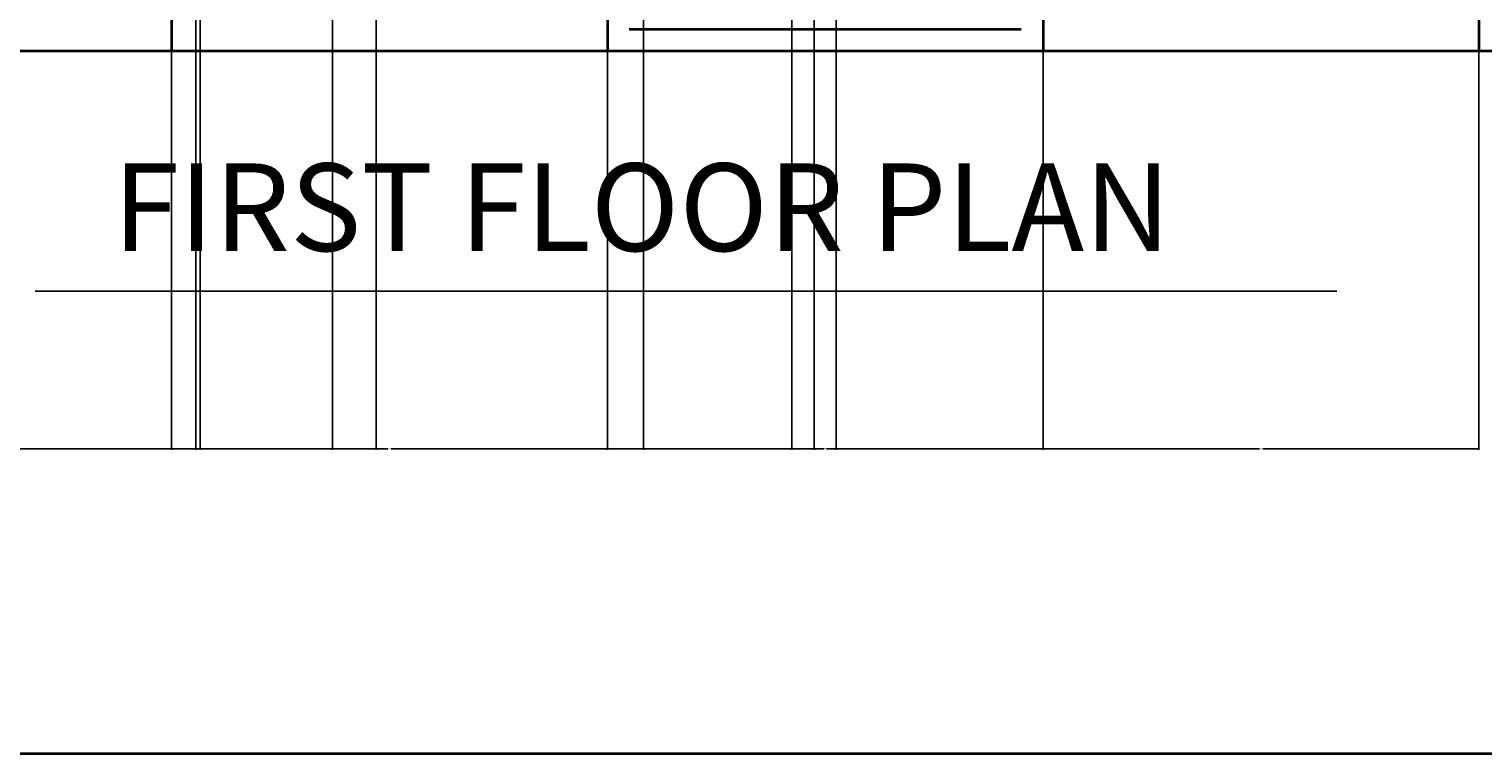
# Model space of a CAD drawing. Units: inches. Extents: x 1721 to 2510, y 1544 to 2360.
# Tile 2 of 10: x 1924 to 2222, y 1544 to 1693. Entities that reach past the tile are written whole.
import ezdxf

# ---------------------------------------------------------------- set-up
doc = ezdxf.new("R2010")
doc.units = ezdxf.units.IN
for name, color, linetype, lineweight in [('A-ANNO-DIMS', 2, 'Continuous', 18), ('A-ANNO-TEXT', 7, 'Continuous', 25), ('A-ANNO-TTLB', 7, 'Continuous', 35), ('A-WALL', 7, 'Continuous', 35)]:
    doc.layers.add(name, color=color, linetype=linetype, lineweight=lineweight)
doc.styles.get("Standard").update_dxf_attribs({"font": 'arial.ttf'})
doc.dimstyles.get("Standard").update_dxf_attribs({"dimtxt": 0.18, "dimasz": 0.18, "dimexe": 0.18, "dimexo": 0.0625, "dimgap": 0.09, "dimtad": 0, "dimtih": 1, "dimtoh": 1, "dimdec": 4, "dimzin": 0, "dimdsep": 46, "dimtxsty": 'Standard', "dimcen": 0.09, "dimadec": 0, "dimazin": 0, "dimtfac": 1, "dimtdec": 4, "dimtofl": 0, "dimtmove": 0, "dimatfit": 3, "dimfxl": 1, "dimtolj": 1, "dimtzin": 0, "dimarcsym": 0})

# ---------------------------------------------------------------- blocks, each defined once
blk = doc.blocks.new('*D42')
at = {"layer": 'A-ANNO-DIMS', "color": 0, "lineweight": -2, "transparency": 16777216}
for p, q in [((1798, 1688.57), (1798, 1606.75)), ((1953, 1688.57), (1953, 1606.75)), ((1798.18, 1606.93), (1875.22, 1606.93)), ((1952.82, 1606.93), (1875.78, 1606.93))]:
    blk.add_line(p, q, dxfattribs=at)
at = {"layer": 'A-ANNO-DIMS', "color": 0, "transparency": 16777216}
for points in [[(1798.18, 1606.96), (1798.18, 1606.9), (1798, 1606.93)], [(1952.82, 1606.96), (1952.82, 1606.9), (1953, 1606.93)]]:
    blk.add_solid(points, dxfattribs=at)
at = {"layer": 'Defpoints', "color": 0, "transparency": 16777216}
for p in [(1798, 1688.63), (1953, 1688.63), (1953, 1606.93)]:
    blk.add_point(p, dxfattribs=at)
at = {"layer": 'A-ANNO-DIMS', "color": 0, "transparency": 16777216, "insert": (1875.5, 1606.93), "char_height": 0.18, "attachment_point": 5}
blk.add_mtext('\\A1;155', dxfattribs=at)
blk = doc.blocks.new('*D43')
at = {"layer": 'A-ANNO-DIMS', "color": 0, "lineweight": -2, "transparency": 16777216}
for p, q in [((1953, 1688.57), (1953, 1606.75)), ((2042.5, 1688.57), (2042.5, 1606.75)), ((1953.18, 1606.93), (1997.43, 1606.93)), ((2042.32, 1606.93), (1998.08, 1606.93))]:
    blk.add_line(p, q, dxfattribs=at)
at = {"layer": 'A-ANNO-DIMS', "color": 0, "transparency": 16777216}
for points in [[(1953.18, 1606.96), (1953.18, 1606.9), (1953, 1606.93)], [(2042.32, 1606.96), (2042.32, 1606.9), (2042.5, 1606.93)]]:
    blk.add_solid(points, dxfattribs=at)
at = {"layer": 'Defpoints', "color": 0, "transparency": 16777216}
for p in [(1953, 1688.63), (2042.5, 1688.63), (2042.5, 1606.93)]:
    blk.add_point(p, dxfattribs=at)
at = {"layer": 'A-ANNO-DIMS', "color": 0, "transparency": 16777216, "insert": (1997.75, 1606.93), "char_height": 0.18, "attachment_point": 5}
blk.add_mtext('\\A1;89.5', dxfattribs=at)
blk = doc.blocks.new('*D44')
at = {"layer": 'A-ANNO-DIMS', "color": 0, "lineweight": -2, "transparency": 16777216}
for p, q in [((2042.5, 1688.57), (2042.5, 1606.75)), ((2132, 1688.57), (2132, 1606.75)), ((2042.68, 1606.93), (2086.93, 1606.93)), ((2131.82, 1606.93), (2087.58, 1606.93))]:
    blk.add_line(p, q, dxfattribs=at)
at = {"layer": 'A-ANNO-DIMS', "color": 0, "transparency": 16777216}
for points in [[(2042.68, 1606.96), (2042.68, 1606.9), (2042.5, 1606.93)], [(2131.82, 1606.96), (2131.82, 1606.9), (2132, 1606.93)]]:
    blk.add_solid(points, dxfattribs=at)
at = {"layer": 'Defpoints', "color": 0, "transparency": 16777216}
for p in [(2042.5, 1688.63), (2132, 1688.63), (2132, 1606.93)]:
    blk.add_point(p, dxfattribs=at)
at = {"layer": 'A-ANNO-DIMS', "color": 0, "transparency": 16777216, "insert": (2087.25, 1606.93), "char_height": 0.18, "attachment_point": 5}
blk.add_mtext('\\A1;89.5', dxfattribs=at)
blk = doc.blocks.new('*D45')
at = {"layer": 'A-ANNO-DIMS', "color": 0, "lineweight": -2, "transparency": 16777216}
for p, q in [((2132, 1688.57), (2132, 1606.75)), ((2221.5, 1688.57), (2221.5, 1606.75)), ((2132.18, 1606.93), (2176.43, 1606.93)), ((2221.32, 1606.93), (2177.08, 1606.93))]:
    blk.add_line(p, q, dxfattribs=at)
at = {"layer": 'A-ANNO-DIMS', "color": 0, "transparency": 16777216}
for points in [[(2132.18, 1606.96), (2132.18, 1606.9), (2132, 1606.93)], [(2221.32, 1606.96), (2221.32, 1606.9), (2221.5, 1606.93)]]:
    blk.add_solid(points, dxfattribs=at)
at = {"layer": 'Defpoints', "color": 0, "transparency": 16777216}
for p in [(2132, 1688.63), (2221.5, 1688.63), (2221.5, 1606.93)]:
    blk.add_point(p, dxfattribs=at)
at = {"layer": 'A-ANNO-DIMS', "color": 0, "transparency": 16777216, "insert": (2176.75, 1606.93), "char_height": 0.18, "attachment_point": 5}
blk.add_mtext('\\A1;89.5', dxfattribs=at)
blk = doc.blocks.new('*D62')
at = {"layer": 'A-ANNO-DIMS', "color": 0, "lineweight": -2, "transparency": 16777216}
for p, q in [((1957.99, 2252.88), (1957.99, 1606.75)), ((1986.02, 2252.88), (1986.02, 1606.75)), ((1958.17, 1606.93), (1971.61, 1606.93)), ((1985.84, 1606.93), (1972.4, 1606.93))]:
    blk.add_line(p, q, dxfattribs=at)
at = {"layer": 'A-ANNO-DIMS', "color": 0, "transparency": 16777216}
for points in [[(1958.17, 1606.96), (1958.17, 1606.9), (1957.99, 1606.93)], [(1985.84, 1606.96), (1985.84, 1606.9), (1986.02, 1606.93)]]:
    blk.add_solid(points, dxfattribs=at)
at = {"layer": 'Defpoints', "color": 0, "transparency": 16777216}
for p in [(1957.99, 2252.94), (1986.02, 2252.94), (1986.02, 1606.93)]:
    blk.add_point(p, dxfattribs=at)
at = {"layer": 'A-ANNO-DIMS', "color": 0, "transparency": 16777216, "insert": (1972.01, 1606.93), "char_height": 0.18, "attachment_point": 5}
blk.add_mtext('\\A1;28.03', dxfattribs=at)
blk = doc.blocks.new('*D63')
at = {"layer": 'A-ANNO-DIMS', "color": 0, "lineweight": -2, "transparency": 16777216}
for p, q in [((1958.89, 2116.38), (1958.89, 1606.75)), ((1995.05, 2116.38), (1995.05, 1606.75)), ((1959.07, 1606.93), (1976.58, 1606.93)), ((1994.87, 1606.93), (1977.36, 1606.93))]:
    blk.add_line(p, q, dxfattribs=at)
at = {"layer": 'A-ANNO-DIMS', "color": 0, "transparency": 16777216}
for points in [[(1959.07, 1606.96), (1959.07, 1606.9), (1958.89, 1606.93)], [(1994.87, 1606.96), (1994.87, 1606.9), (1995.05, 1606.93)]]:
    blk.add_solid(points, dxfattribs=at)
at = {"layer": 'Defpoints', "color": 0, "transparency": 16777216}
for p in [(1958.89, 2116.44), (1995.05, 2116.44), (1995.05, 1606.93)]:
    blk.add_point(p, dxfattribs=at)
at = {"layer": 'A-ANNO-DIMS', "color": 0, "transparency": 16777216, "insert": (1976.97, 1606.93), "char_height": 0.18, "attachment_point": 5}
blk.add_mtext('\\A1;36.16', dxfattribs=at)
blk = doc.blocks.new('*D64')
at = {"layer": 'A-ANNO-DIMS', "color": 0, "lineweight": -2, "transparency": 16777216}
for p, q in [((2049.89, 1986.57), (2049.89, 1606.75)), ((2080.39, 1986.57), (2080.39, 1606.75)), ((2050.07, 1606.93), (2064.81, 1606.93)), ((2080.21, 1606.93), (2065.46, 1606.93))]:
    blk.add_line(p, q, dxfattribs=at)
at = {"layer": 'A-ANNO-DIMS', "color": 0, "transparency": 16777216}
for points in [[(2050.07, 1606.96), (2050.07, 1606.9), (2049.89, 1606.93)], [(2080.21, 1606.96), (2080.21, 1606.9), (2080.39, 1606.93)]]:
    blk.add_solid(points, dxfattribs=at)
at = {"layer": 'Defpoints', "color": 0, "transparency": 16777216}
for p in [(2049.89, 1986.63), (2080.39, 1986.63), (2080.39, 1606.93)]:
    blk.add_point(p, dxfattribs=at)
at = {"layer": 'A-ANNO-DIMS', "color": 0, "transparency": 16777216, "insert": (2065.14, 1606.93), "char_height": 0.18, "attachment_point": 5}
blk.add_mtext('\\A1;30.5', dxfattribs=at)
blk = doc.blocks.new('*D65')
at = {"layer": 'A-ANNO-DIMS', "color": 0, "lineweight": -2, "transparency": 16777216}
for p, q in [((2085, 2116.38), (2085, 1606.75)), ((2089.5, 2116.38), (2089.5, 1606.75)), ((2085.18, 1606.93), (2086.99, 1606.93)), ((2089.32, 1606.93), (2087.51, 1606.93))]:
    blk.add_line(p, q, dxfattribs=at)
at = {"layer": 'A-ANNO-DIMS', "color": 0, "transparency": 16777216}
for points in [[(2085.18, 1606.96), (2085.18, 1606.9), (2085, 1606.93)], [(2089.32, 1606.96), (2089.32, 1606.9), (2089.5, 1606.93)]]:
    blk.add_solid(points, dxfattribs=at)
at = {"layer": 'Defpoints', "color": 0, "transparency": 16777216}
for p in [(2085, 2116.44), (2089.5, 2116.44), (2089.5, 1606.93)]:
    blk.add_point(p, dxfattribs=at)
at = {"layer": 'A-ANNO-DIMS', "color": 0, "transparency": 16777216, "insert": (2087.25, 1606.93), "char_height": 0.18, "attachment_point": 5}
blk.add_mtext('\\A1;4.5', dxfattribs=at)
blk = doc.blocks.new('*D67')
at = {"layer": 'A-ANNO-DIMS', "color": 0, "lineweight": -2, "transparency": 16777216}
for p, q in [((2042.44, 1725.13), (1765.42, 1725.13)), ((1765.6, 1724.95), (1765.6, 1707.06)), ((1765.6, 1688.81), (1765.6, 1706.7)), ((2042.44, 1688.63), (1765.42, 1688.63))]:
    blk.add_line(p, q, dxfattribs=at)
at = {"layer": 'A-ANNO-DIMS', "color": 0, "transparency": 16777216}
for points in [[(1765.57, 1724.95), (1765.63, 1724.95), (1765.6, 1725.13)], [(1765.57, 1688.81), (1765.63, 1688.81), (1765.6, 1688.63)]]:
    blk.add_solid(points, dxfattribs=at)
at = {"layer": 'Defpoints', "color": 0, "transparency": 16777216}
for p in [(1765.6, 1725.13), (2042.5, 1725.13), (2042.5, 1688.63)]:
    blk.add_point(p, dxfattribs=at)
at = {"layer": 'A-ANNO-DIMS', "color": 0, "transparency": 16777216, "insert": (1765.6, 1706.88), "char_height": 0.18, "attachment_point": 5}
blk.add_mtext('\\A1;36.5', dxfattribs=at)

msp = doc.modelspace()

# ---------------------------------------------------------------- linework, layer by layer
at = {"layer": 'A-ANNO-TEXT'}
msp.add_line((1924.9747, 1639.3297), (2192.2869, 1639.3297), dxfattribs=at)
at = {"layer": 'A-ANNO-TTLB'}
msp.add_lwpolyline([(1721.1268, 2360.2177), (2509.707, 2360.2177), (2509.707, 1544.3037), (1721.1268, 1544.3037)], close=True, dxfattribs=at)
at = {"layer": 'A-WALL'}
for p, q in [((1953.0024, 1829.1298), (1953.0024, 1688.6298)), ((2042.5024, 1725.1298), (2042.5024, 1688.6298)), ((2132.0024, 1725.1298), (2132.0024, 1688.6298)), ((2221.5024, 1725.1298), (2221.5024, 1688.6298)), ((2047.0024, 1693.1298), (2127.5024, 1693.1298)), ((1798.0024, 1688.6298), (2376.5024, 1688.6298))]:
    msp.add_line(p, q, dxfattribs=at)

# ---------------------------------------------------------------- texts
at = {"layer": 'A-ANNO-TEXT', "insert": (1940.9862, 1665.5549), "char_height": 18, "attachment_point": 1}
msp.add_mtext_dynamic_manual_height_columns('FIRST FLOOR PLAN', width=420.795796, gutter_width=12.5, heights=[0], dxfattribs=at)

# ---------------------------------------------------------------- dimensions: what is measured, and where the dimension line sits
at = {"layer": 'A-ANNO-DIMS'}
for base, p1, p2, override, picture, middle in [((1986.0213, 1606.9297), (1957.9903, 2252.9416), (1986.0213, 2252.9416), {"dimdec": 2, "dimlfac": 1, "dimrnd": 0, "dimzin": 0, "dimdsep": 46, "dimlunit": 2}, '*D62', (1972.0058, 1606.9297)), ((1995.0512, 1606.9297), (1958.8889, 2116.4416), (1995.0512, 2116.4416), {"dimdec": 2, "dimlfac": 1, "dimrnd": 0, "dimzin": 0, "dimdsep": 46, "dimlunit": 2}, '*D63', (1976.97, 1606.9297)), ((2089.5024, 1606.9297), (2085.0024, 2116.4416), (2089.5024, 2116.4416), {"dimdec": 1, "dimlfac": 1, "dimrnd": 0, "dimzin": 0, "dimdsep": 46, "dimlunit": 2}, '*D65', (2087.2524, 1606.9297)), ((2080.3854, 1606.9297), (2049.8856, 1986.6298), (2080.3854, 1986.6298), {"dimdec": 1, "dimlfac": 1, "dimrnd": 0, "dimzin": 0, "dimdsep": 46, "dimlunit": 2}, '*D64', (2065.1355, 1606.9297)), ((1953.0024, 1606.9297), (1798.0024, 1688.6298), (1953.0024, 1688.6298), {"dimdec": 0, "dimlfac": 1, "dimrnd": 0, "dimzin": 0, "dimdsep": 46, "dimlunit": 2}, '*D42', (1875.5024, 1606.9297)), ((2042.5024, 1606.9297), (1953.0024, 1688.6298), (2042.5024, 1688.6298), {"dimdec": 1, "dimlfac": 1, "dimrnd": 0, "dimzin": 0, "dimdsep": 46, "dimlunit": 2}, '*D43', (1997.7524, 1606.9297)), ((2132.0024, 1606.9297), (2042.5024, 1688.6298), (2132.0024, 1688.6298), {"dimdec": 1, "dimlfac": 1, "dimrnd": 0, "dimzin": 0, "dimdsep": 46, "dimlunit": 2}, '*D44', (2087.2524, 1606.9297)), ((2221.5024, 1606.9297), (2132.0024, 1688.6298), (2221.5024, 1688.6298), {"dimdec": 1, "dimlfac": 1, "dimrnd": 0, "dimzin": 0, "dimdsep": 46, "dimlunit": 2}, '*D45', (2176.7524, 1606.9297))]:
    dim = msp.add_linear_dim(base=base, p1=p1, p2=p2, dimstyle='Standard', override=override, dxfattribs=at)
    dim.commit()
    dim.dimension.update_dxf_attribs({"geometry": picture, "text_midpoint": middle})
dim = msp.add_linear_dim(base=(1765.6024, 1725.1298), p1=(2042.5024, 1688.6298), p2=(2042.5024, 1725.1298), angle=90, dimstyle='Standard', override={"dimdec": 1, "dimlfac": 1, "dimrnd": 0, "dimzin": 0, "dimdsep": 46, "dimlunit": 2}, dxfattribs=at)
dim.commit()
dim.dimension.update_dxf_attribs({"geometry": '*D67', "text_midpoint": (1765.6024, 1706.8798)})

doc.saveas('drawing.dxf')
